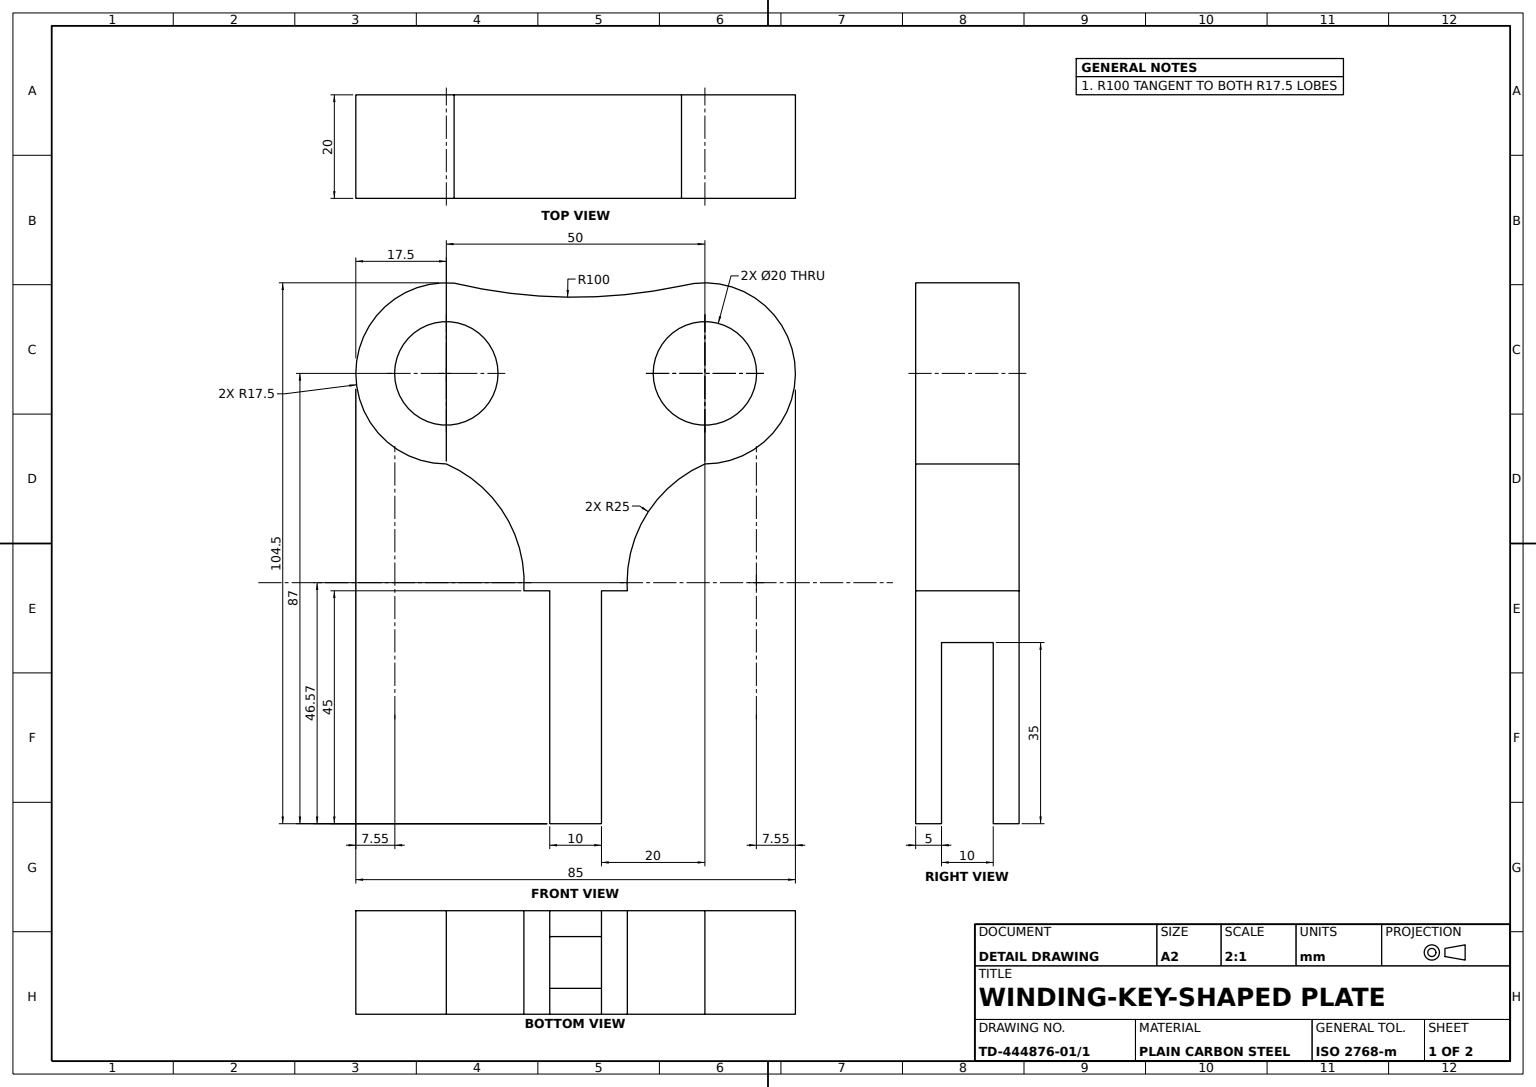
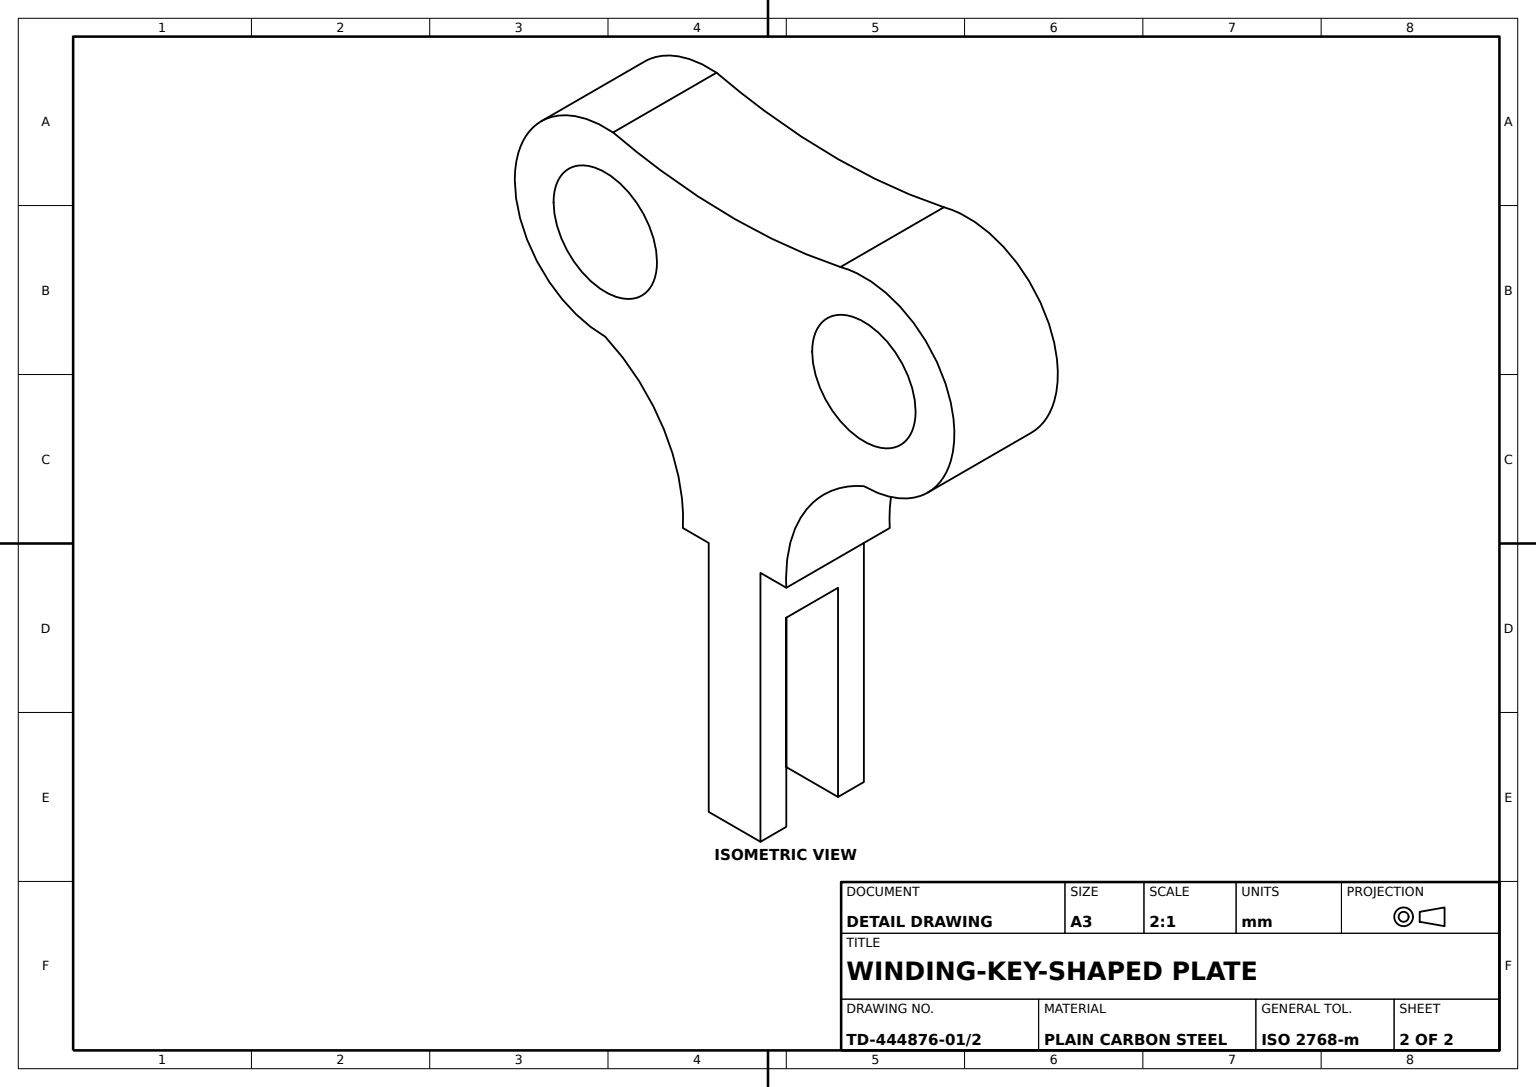
SolidWorks part; units mm, degrees
material "Plain Carbon Steel"
ref_plane "Front Plane" through (0, 0, 0) normal (0, 0, 1) x (1, 0, 0)
ref_plane "Top Plane" through (0, 0, 0) normal (0, 1, 0) x (1, 0, 0)
ref_plane "Right Plane" through (0, 0, 0) normal (1, 0, 0) x (0, 0, -1)
sketch "Key Profile Sketch" plane through (0, 0, 0) normal (0, 0, 1) x (1, 0, 0)
  line L2 (25, -87) -> (30, -87)
  line L3 (25, -87) -> (20, -87)
  line L4 (20, -87) -> (20, -42)
  line L5 (20, -42) -> (15, -42)
  line L6 (30, -87) -> (30, -42)
  line L7 (30, -42) -> (35, -42)
  arc A0 (50, -17.5) -> (45.4753, 16.905) centre (50, 0) ccw
  arc A1 (1.506, 17.4351) -> (0, -17.5) centre (0, 0) ccw
  arc A2 (1.506, 17.4351) -> (45.4753, 16.905) centre (24.6667, 114.716) ccw
  arc A3 (15, -42) -> (0, -17.5) centre (-9.9509, -40.4342) ccw
  arc A4 (35, -42) -> (50, -17.5) centre (59.9509, -40.4342) cw
  dimension "D1" = 35
  dimension "D2" = 35
  dimension "D3" = 17.5
  dimension "D4" = 100
  dimension "D5" = 25
  dimension "D6" = 4.6667
  dimension "D7" = 5
  dimension "D8" = 25.4753
  dimension "D9" = 30
  dimension "D10" = 39.9509
  dimension "D11" = 45
extrude "Key Body" add sketch "Key Profile Sketch" along normal blind 20
sketch "Shank Slot Sketch" plane through (30, 0, 0) normal (1, 0, 0) x (0, 0, -1)
  line L0 (-20, -87) -> (-15, -87)
  line L1 (-20, -87) -> (0, -87) construction
  line L2 (-15, -87) -> (-15, -52)
  line L3 (-15, -52) -> (-5, -52)
  line L4 (-5, -52) -> (-5, -87)
  line L5 (-5, -87) -> (-15, -87)
  line L6 (0, -87) -> (0, -42) construction
  line L7 (-20, -42) -> (0, -42) construction
  line M4 (-20, -87) -> (0, -87)
  dimension "D1" = 5
  dimension "D2" = 15
  dimension "D3" = 10
extrude "Shank Slot" cut sketch "Shank Slot Sketch" against normal blind 20 contours L4 L3 L2 M4
sketch "Grip Holes Sketch" plane through (0, 0, 20) normal (0, 0, 1) x (1, 0, 0)
  circle A0 centre (0, 0) radius 10
  circle A1 centre (50, 0) radius 10
  dimension "D1" = 20
  dimension "D2" = 20
  dimension "D3" = 20
extrude "Grip Holes 2xØ20" cut sketch "Grip Holes Sketch" against normal blind 20
